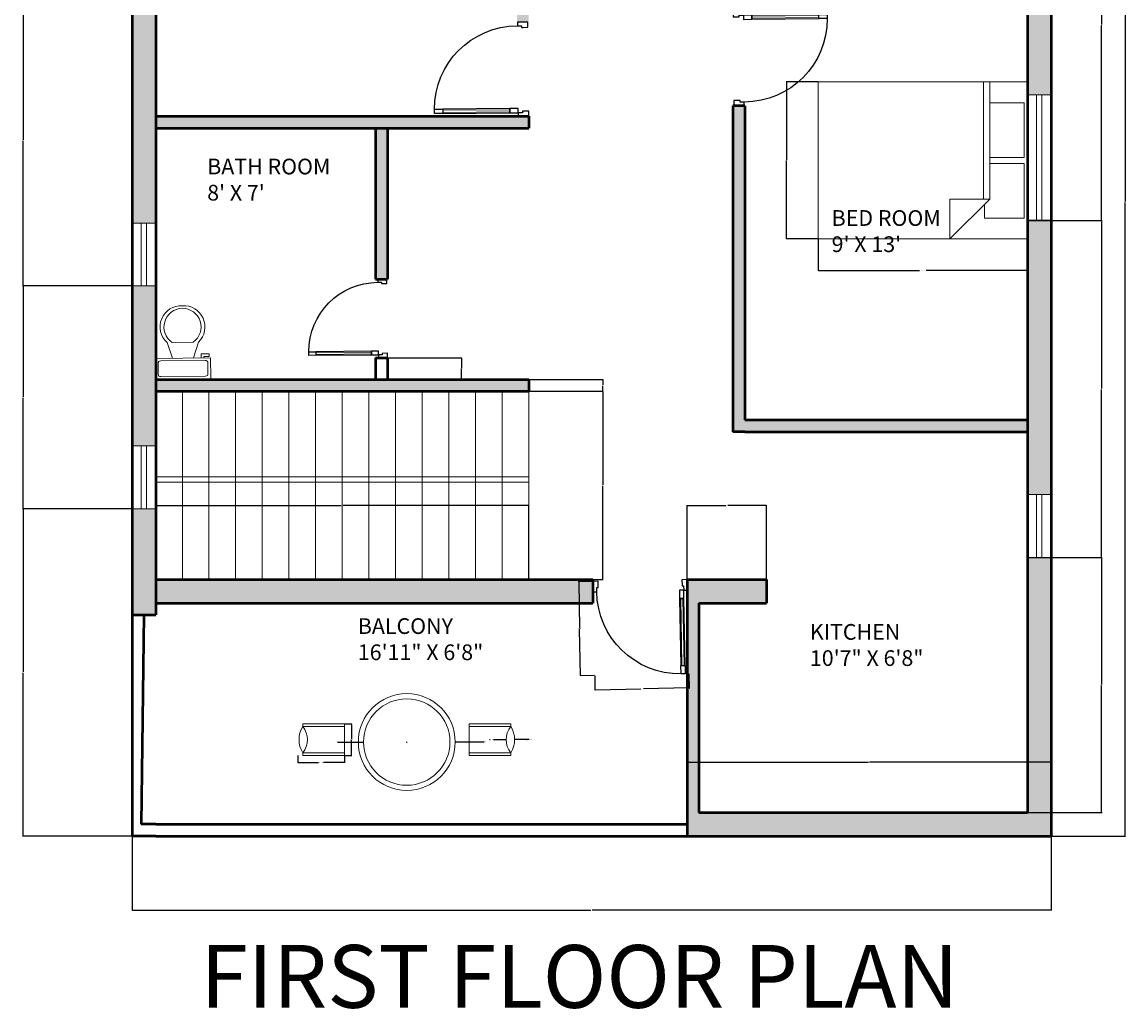
# Model space of a CAD drawing. Units: inches. Extents: x 5704 to 6126, y 2544 to 3123.
# Tile 1 of 2: x 5704 to 6126, y 2544 to 2921. Entities that reach past the tile are written whole.
import ezdxf

# ---------------------------------------------------------------- set-up
doc = ezdxf.new("R2010")
doc.units = ezdxf.units.IN
for name, color, linetype, lineweight in [('A-ANNO-DIMS', 2, 'Continuous', 18), ('A-ANNO-TEXT', 7, 'Continuous', 35), ('A-AREA-IDEN', 7, 'Continuous', 18), ('A-Door', 150, 'Continuous', 25), ('A-FLOR-FIXT', 9, 'Continuous', 18), ('A-FLOR-STRS', 7, 'Continuous', 18), ('A-FURN', 8, 'Continuous', 18), ('A-Glaz', 92, 'Continuous', 18), ('A-WALL', 7, 'Continuous', 50)]:
    doc.layers.add(name, color=color, linetype=linetype, lineweight=lineweight)
doc.layers.add('A-WALL-PATT', color=18, linetype='Continuous', lineweight=13, true_color=0x000000)
doc.styles.get("Standard").update_dxf_attribs({"font": 'arial.ttf'})
doc.dimstyles.get("Standard").update_dxf_attribs({"dimtxt": 0.18, "dimasz": 0.18, "dimexe": 0.18, "dimexo": 0.0625, "dimgap": 0.09, "dimtad": 0, "dimtih": 1, "dimtoh": 1, "dimdec": 4, "dimzin": 0, "dimdsep": 46, "dimtxsty": 'Standard', "dimcen": 0.09, "dimadec": 0, "dimazin": 0, "dimtfac": 1, "dimtdec": 4, "dimtofl": 0, "dimtmove": 0, "dimatfit": 3, "dimfxl": 1, "dimtolj": 1, "dimtzin": 0, "dimarcsym": 0})

# ---------------------------------------------------------------- blocks, each defined once
blk = doc.blocks.new('A$C61230BBC')
blk.add_lwpolyline([(825, 180), (825, 820), (865, 820), (865, 180)], close=True)
blk.add_arc((830, 105), 795, 90.3603, 180.3603)
at = {"layer": 'A-Door'}
for points in [[(825, 900), (825, 820), (865, 820), (865, 900)], [(825, 100), (825, 180), (865, 180), (865, 100)], [(35, 100), (35, 60), (50, 60), (50, 50), (50, 0), (0, 0), (0, 100)], [(865, 100), (900, 100), (900, 0), (850, 0), (850, 50), (850, 60), (865, 60)]]:
    blk.add_lwpolyline(points, close=True, dxfattribs=at)
at = {"layer": 'A-Glaz'}
blk.add_lwpolyline([(835, 180), (835, 820), (855, 820), (855, 180)], close=True, dxfattribs=at)
blk = doc.blocks.new('*U3')
for p, q in [((9.5, -6), (9.5, -2)), ((-8, -8.5), (-8, -8)), ((-7, -8), (-7, -9.5)), ((-4, -8), (-6, -14)), ((4, -8), (6, -14)), ((-10, -8.5), (-8, -8.5)), ((-10, -9.5), (-10, -8.5)), ((-7, -9.5), (-10, -9.5)), ((4, -14), (-4, -14))]:
    blk.add_line(p, q)
blk.add_lwpolyline([(10.5, -8), (10.5, 0), (-10.5, 0), (-10.5, -8)], close=True)
for points in [[(-9.5, -2), (-9.5, -6)], [(8.5, -1), (-8.5, -1)], [(-8.5, -7), (8.5, -7)]]:
    blk.add_lwpolyline(points)
for centre, radius, start, end in [((-8.625, -1.875), 0.8839, 81.8699, 188.1301), ((8.625, -1.875), 0.8839, 351.8699, 98.1301), ((-8.625, -6.125), 0.8839, 171.869898, 278.1301), ((8.625, -6.125), 0.8839, 261.8699, 8.1301), ((-0.4772, -19.9188), 8.0953, 133.01722, 273.38), ((0.0374, -19.8731), 7.127, 124.50543, 269.7), ((-0.0373, -19.8731), 7.127, 270.3, 55.4946), ((0.4773, -19.9188), 8.0953, 266.62, 46.9828)]:
    blk.add_arc(centre, radius, start, end)
blk = doc.blocks.new('Bed - Queen')
for p, q in [((0, -80.00003), (0, 0)), ((0, 0), (59.99999, 0)), ((59.99999, 0), (59.99999, -80.00003)), ((7.99999, -1.2), (28.79998, -1.2)), ((7.99999, -14.4), (7.99999, -1.2)), ((28.79998, -1.2), (28.79998, -14.4)), ((31.19999, -1.2), (51.99999, -1.2)), ((31.19999, -14.4), (31.19999, -1.2)), ((51.99999, -1.2), (51.99999, -16.4)), ((0, -14.4), (44.8, -14.4)), ((44.8, -16.8), (0, -16.8)), ((59.99999, -29.6), (44.8, -14.4)), ((44.8, -14.4), (44.8, -29.6)), ((51.99999, -16.4), (46.79936, -16.4)), ((44.8, -29.6), (59.99999, -29.6)), ((59.99999, -80.00003), (0, -80.00003))]:
    blk.add_line(p, q)
blk = doc.blocks.new('WIN-24IN')
for p, q in [((0, 9), (0, 0)), ((24, 9), (24, 0)), ((0, 5.5), (24, 5.5)), ((0, 3.5), (24, 3.5))]:
    blk.add_line(p, q)
blk = doc.blocks.new('WIN-48IN')
for p, q in [((0, 48), (9, 48)), ((3.5, 48), (3.5, 0)), ((5.5, 48), (5.5, 0)), ((5.5, 48), (5.5, 0)), ((0, 0), (9, 0))]:
    blk.add_line(p, q)
blk = doc.blocks.new('CHAIR-BALCONY')
for p, q in [((0, 12), (15.92, 12)), ((0, 12), (0, 0)), ((15.92, 11), (0, 11)), ((15.92, 12), (15.92, 11)), ((0, 1), (15.92, 1)), ((15.92, 0), (0, 0)), ((15.92, 1), (15.92, 0))]:
    blk.add_line(p, q)
for centre, radius, start, end in [((22.11, 6), 7.96, 141.1063, 218.8937), ((7.96, 6), 9.4, 327.8579, 32.1421)]:
    blk.add_arc(centre, radius, start, end)
blk = doc.blocks.new('*D10')
at = {"layer": 'A-ANNO-DIMS', "color": 0, "lineweight": -2, "transparency": 16777216}
for p, q in [((5922.38, 2706.94), (5916.86, 2706.84)), ((5917.05, 2706.66), (5917.38, 2689.03)), ((5917.72, 2671.03), (5917.38, 2688.66)), ((5923.06, 2670.95), (5917.54, 2670.85))]:
    blk.add_line(p, q, dxfattribs=at)
at = {"layer": 'A-ANNO-DIMS', "color": 0, "transparency": 16777216}
for points in [[(5917.08, 2706.66), (5917.02, 2706.66), (5917.04, 2706.84)], [(5917.75, 2671.03), (5917.69, 2671.03), (5917.72, 2670.85)]]:
    blk.add_solid(points, dxfattribs=at)
at = {"layer": 'Defpoints', "color": 0, "transparency": 16777216}
for p in [(5922.44, 2706.94), (5917.72, 2670.85), (5923.12, 2670.95)]:
    blk.add_point(p, dxfattribs=at)
at = {"layer": 'A-ANNO-DIMS', "color": 0, "transparency": 16777216, "insert": (5917.38, 2688.85), "char_height": 0.18, "attachment_point": 5}
blk.add_mtext('\\A1;DOOR 36 TYP.', dxfattribs=at)
blk = doc.blocks.new('*D11')
at = {"layer": 'A-ANNO-DIMS', "color": 0, "lineweight": -2, "transparency": 16777216}
for p, q in [((5923.12, 2670.89), (5923.22, 2665.37)), ((5959.11, 2671.56), (5959.22, 2666.05)), ((5923.4, 2665.55), (5940.69, 2665.88)), ((5959.03, 2666.22), (5941.74, 2665.9))]:
    blk.add_line(p, q, dxfattribs=at)
at = {"layer": 'A-ANNO-DIMS', "color": 0, "transparency": 16777216}
for points in [[(5923.4, 2665.58), (5923.4, 2665.52), (5923.22, 2665.55)], [(5959.03, 2666.25), (5959.03, 2666.19), (5959.21, 2666.23)]]:
    blk.add_solid(points, dxfattribs=at)
at = {"layer": 'Defpoints', "color": 0, "transparency": 16777216}
for p in [(5923.12, 2670.95), (5959.11, 2671.62), (5959.21, 2666.23)]:
    blk.add_point(p, dxfattribs=at)
at = {"layer": 'A-ANNO-DIMS', "color": 0, "transparency": 16777216, "insert": (5941.22, 2665.89), "char_height": 0.18, "attachment_point": 5}
blk.add_mtext('\\A1;36 TYP.', dxfattribs=at)
blk = doc.blocks.new('*D16')
at = {"layer": 'A-ANNO-DIMS', "color": 0, "lineweight": -2, "transparency": 16777216}
for p, q in [((6008.44, 2837.68), (6008.44, 2825.56)), ((6088.44, 2837.68), (6088.44, 2825.56)), ((6008.62, 2825.74), (6047.13, 2825.74)), ((6088.26, 2825.74), (6049.74, 2825.74))]:
    blk.add_line(p, q, dxfattribs=at)
at = {"layer": 'A-ANNO-DIMS', "color": 0, "transparency": 16777216}
for points in [[(6008.62, 2825.77), (6008.62, 2825.71), (6008.44, 2825.74)], [(6088.26, 2825.77), (6088.26, 2825.71), (6088.44, 2825.74)]]:
    blk.add_solid(points, dxfattribs=at)
at = {"layer": 'Defpoints', "color": 0, "transparency": 16777216}
for p in [(6008.44, 2837.74), (6088.44, 2837.74), (6088.44, 2825.74)]:
    blk.add_point(p, dxfattribs=at)
at = {"layer": 'A-ANNO-DIMS', "color": 0, "transparency": 16777216, "insert": (6048.44, 2825.74), "char_height": 0.18, "attachment_point": 5}
blk.add_mtext('\\A1;QUEEN BED 80 TYP.', dxfattribs=at)
blk = doc.blocks.new('*D17')
at = {"layer": 'A-ANNO-DIMS', "color": 0, "lineweight": -2, "transparency": 16777216}
for p, q in [((6008.37, 2897.74), (5996.26, 2897.74)), ((5996.44, 2897.56), (5996.44, 2867.92)), ((5996.44, 2837.92), (5996.44, 2867.56)), ((6008.37, 2837.74), (5996.26, 2837.74))]:
    blk.add_line(p, q, dxfattribs=at)
at = {"layer": 'A-ANNO-DIMS', "color": 0, "transparency": 16777216}
for points in [[(5996.41, 2897.56), (5996.47, 2897.56), (5996.44, 2897.74)], [(5996.41, 2837.92), (5996.47, 2837.92), (5996.44, 2837.74)]]:
    blk.add_solid(points, dxfattribs=at)
at = {"layer": 'Defpoints', "color": 0, "transparency": 16777216}
for p in [(6008.44, 2897.74), (5996.44, 2837.74), (6008.44, 2837.74)]:
    blk.add_point(p, dxfattribs=at)
at = {"layer": 'A-ANNO-DIMS', "color": 0, "transparency": 16777216, "insert": (5996.44, 2867.74), "char_height": 0.18, "attachment_point": 5}
blk.add_mtext('\\A1;60 TYP.', dxfattribs=at)
blk = doc.blocks.new('*D18')
at = {"layer": 'A-ANNO-DIMS', "color": 0, "lineweight": -2, "transparency": 16777216}
for p, q in [((5809.71, 2640.4), (5809.71, 2637.6)), ((5827.55, 2640.4), (5827.55, 2637.6)), ((5809.89, 2637.78), (5817.68, 2637.78)), ((5827.37, 2637.78), (5819.58, 2637.78))]:
    blk.add_line(p, q, dxfattribs=at)
at = {"layer": 'A-ANNO-DIMS', "color": 0, "transparency": 16777216}
for points in [[(5809.89, 2637.81), (5809.89, 2637.75), (5809.71, 2637.78)], [(5827.37, 2637.81), (5827.37, 2637.75), (5827.55, 2637.78)]]:
    blk.add_solid(points, dxfattribs=at)
at = {"layer": 'Defpoints', "color": 0, "transparency": 16777216}
for p in [(5809.71, 2640.46), (5827.55, 2640.46), (5809.71, 2637.78)]:
    blk.add_point(p, dxfattribs=at)
at = {"layer": 'A-ANNO-DIMS', "color": 0, "transparency": 16777216, "insert": (5818.63, 2637.78), "char_height": 0.18, "attachment_point": 5}
blk.add_mtext('\\A1;CHAIR 18 TYP.', dxfattribs=at)
blk = doc.blocks.new('*D19')
at = {"layer": 'A-ANNO-DIMS', "color": 0, "lineweight": -2, "transparency": 16777216}
for p, q in [((5827.61, 2652.46), (5830.4, 2652.46)), ((5830.22, 2652.28), (5830.22, 2646.64)), ((5830.22, 2640.64), (5830.22, 2646.28)), ((5827.61, 2640.46), (5830.4, 2640.46))]:
    blk.add_line(p, q, dxfattribs=at)
at = {"layer": 'A-ANNO-DIMS', "color": 0, "transparency": 16777216}
for points in [[(5830.19, 2652.28), (5830.25, 2652.28), (5830.22, 2652.46)], [(5830.19, 2640.64), (5830.25, 2640.64), (5830.22, 2640.46)]]:
    blk.add_solid(points, dxfattribs=at)
at = {"layer": 'Defpoints', "color": 0, "transparency": 16777216}
for p in [(5827.55, 2652.46), (5827.55, 2640.46), (5830.22, 2640.46)]:
    blk.add_point(p, dxfattribs=at)
at = {"layer": 'A-ANNO-DIMS', "color": 0, "transparency": 16777216, "insert": (5830.22, 2646.46), "char_height": 0.18, "attachment_point": 5}
blk.add_mtext('\\A1;12 TYP.', dxfattribs=at)
blk = doc.blocks.new('*D20')
at = {"layer": 'A-ANNO-DIMS', "color": 0, "lineweight": -2, "transparency": 16777216}
for p, q in [((5746.436687, 2609.555742), (5746.436687, 2581.138242)), ((6097.436687, 2609.555742), (6097.436687, 2581.138242)), ((5746.616687, 2581.318242), (5921.665275, 2581.318242)), ((6097.256687, 2581.318242), (5922.208099, 2581.318242))]:
    blk.add_line(p, q, dxfattribs=at)
at = {"layer": 'A-ANNO-DIMS', "color": 0, "transparency": 16777216}
for points in [[(5746.616687, 2581.348242), (5746.616687, 2581.288242), (5746.436687, 2581.318242)], [(6097.256687, 2581.348242), (6097.256687, 2581.288242), (6097.436687, 2581.318242)]]:
    blk.add_solid(points, dxfattribs=at)
at = {"layer": 'Defpoints', "color": 0, "transparency": 16777216}
for p in [(5746.436687, 2609.618242), (6097.436687, 2609.618242), (6097.436687, 2581.318242)]:
    blk.add_point(p, dxfattribs=at)
at = {"layer": 'A-ANNO-DIMS', "color": 0, "transparency": 16777216, "insert": (5921.936687, 2581.318242), "char_height": 0.18, "attachment_point": 5}
blk.add_mtext('\\A1;351', dxfattribs=at)
blk = doc.blocks.new('*D21')
at = {"layer": 'A-ANNO-DIMS', "color": 0, "lineweight": -2, "transparency": 16777216}
for p, q in [((6097.5, 3094.12), (6125.92, 3094.12)), ((6125.74, 3093.94), (6125.74, 2852.05)), ((6125.74, 2609.8), (6125.74, 2851.69)), ((6097.5, 2609.62), (6125.92, 2609.62))]:
    blk.add_line(p, q, dxfattribs=at)
at = {"layer": 'A-ANNO-DIMS', "color": 0, "transparency": 16777216}
for points in [[(6125.71, 3093.94), (6125.77, 3093.94), (6125.74, 3094.12)], [(6125.71, 2609.8), (6125.77, 2609.8), (6125.74, 2609.62)]]:
    blk.add_solid(points, dxfattribs=at)
at = {"layer": 'Defpoints', "color": 0, "transparency": 16777216}
for p in [(6097.44, 3094.12), (6125.74, 3094.12), (6097.44, 2609.62)]:
    blk.add_point(p, dxfattribs=at)
at = {"layer": 'A-ANNO-DIMS', "color": 0, "transparency": 16777216, "insert": (6125.74, 2851.87), "char_height": 0.18, "attachment_point": 5}
blk.add_mtext('\\A1;484.5', dxfattribs=at)
blk = doc.blocks.new('*D24')
at = {"layer": 'A-ANNO-DIMS', "color": 0, "lineweight": -2, "transparency": 16777216}
for p, q in [((5746.37, 2734.68), (5704.59, 2734.68)), ((5704.77, 2734.5), (5704.77, 2672.33)), ((5704.77, 2609.8), (5704.77, 2671.97)), ((5746.37, 2609.62), (5704.59, 2609.62))]:
    blk.add_line(p, q, dxfattribs=at)
at = {"layer": 'A-ANNO-DIMS', "color": 0, "transparency": 16777216}
for points in [[(5704.74, 2734.5), (5704.8, 2734.5), (5704.77, 2734.68)], [(5704.74, 2609.8), (5704.8, 2609.8), (5704.77, 2609.62)]]:
    blk.add_solid(points, dxfattribs=at)
at = {"layer": 'Defpoints', "color": 0, "transparency": 16777216}
for p in [(5704.77, 2734.68), (5746.44, 2734.68), (5746.44, 2609.62)]:
    blk.add_point(p, dxfattribs=at)
at = {"layer": 'A-ANNO-DIMS', "color": 0, "transparency": 16777216, "insert": (5704.77, 2672.15), "char_height": 0.18, "attachment_point": 5}
blk.add_mtext('\\A1;125.06', dxfattribs=at)
blk = doc.blocks.new('*D25')
at = {"layer": 'A-ANNO-DIMS', "color": 0, "lineweight": -2, "transparency": 16777216}
for p, q in [((5746.37, 2819.8), (5704.59, 2819.8)), ((5704.77, 2819.62), (5704.77, 2777.42)), ((5704.77, 2734.86), (5704.77, 2777.06)), ((5746.37, 2734.68), (5704.59, 2734.68))]:
    blk.add_line(p, q, dxfattribs=at)
at = {"layer": 'A-ANNO-DIMS', "color": 0, "transparency": 16777216}
for points in [[(5704.74, 2819.62), (5704.8, 2819.62), (5704.77, 2819.8)], [(5704.74, 2734.86), (5704.8, 2734.86), (5704.77, 2734.68)]]:
    blk.add_solid(points, dxfattribs=at)
at = {"layer": 'Defpoints', "color": 0, "transparency": 16777216}
for p in [(5704.77, 2819.8), (5746.44, 2819.8), (5746.44, 2734.68)]:
    blk.add_point(p, dxfattribs=at)
at = {"layer": 'A-ANNO-DIMS', "color": 0, "transparency": 16777216, "insert": (5704.77, 2777.24), "char_height": 0.18, "attachment_point": 5}
blk.add_mtext('\\A1;85.12', dxfattribs=at)
blk = doc.blocks.new('*D26')
at = {"layer": 'A-ANNO-DIMS', "color": 0, "lineweight": -2, "transparency": 16777216}
for p, q in [((5746.37, 2931.06), (5704.59, 2931.06)), ((5704.77, 2930.88), (5704.77, 2875.61)), ((5704.77, 2819.98), (5704.77, 2875.25)), ((5746.37, 2819.8), (5704.59, 2819.8))]:
    blk.add_line(p, q, dxfattribs=at)
at = {"layer": 'A-ANNO-DIMS', "color": 0, "transparency": 16777216}
for points in [[(5704.74, 2930.88), (5704.8, 2930.88), (5704.77, 2931.06)], [(5704.74, 2819.98), (5704.8, 2819.98), (5704.77, 2819.8)]]:
    blk.add_solid(points, dxfattribs=at)
at = {"layer": 'Defpoints', "color": 0, "transparency": 16777216}
for p in [(5704.77, 2931.06), (5746.44, 2931.06), (5746.44, 2819.8)]:
    blk.add_point(p, dxfattribs=at)
at = {"layer": 'A-ANNO-DIMS', "color": 0, "transparency": 16777216, "insert": (5704.77, 2875.43), "char_height": 0.18, "attachment_point": 5}
blk.add_mtext('\\A1;111.27', dxfattribs=at)
blk = doc.blocks.new('*D27')
at = {"layer": 'A-ANNO-DIMS', "color": 0, "lineweight": -2, "transparency": 16777216}
for p, q in [((6088.5, 2716.09), (6116.92, 2716.09)), ((6116.74, 2715.91), (6116.74, 2667.54)), ((6116.74, 2618.8), (6116.74, 2667.17)), ((6088.5, 2618.62), (6116.92, 2618.62))]:
    blk.add_line(p, q, dxfattribs=at)
at = {"layer": 'A-ANNO-DIMS', "color": 0, "transparency": 16777216}
for points in [[(6116.71, 2715.91), (6116.77, 2715.91), (6116.74, 2716.09)], [(6116.71, 2618.8), (6116.77, 2618.8), (6116.74, 2618.62)]]:
    blk.add_solid(points, dxfattribs=at)
at = {"layer": 'Defpoints', "color": 0, "transparency": 16777216}
for p in [(6088.44, 2716.09), (6088.44, 2618.62), (6116.74, 2618.62)]:
    blk.add_point(p, dxfattribs=at)
at = {"layer": 'A-ANNO-DIMS', "color": 0, "transparency": 16777216, "insert": (6116.74, 2667.36), "char_height": 0.18, "attachment_point": 5}
blk.add_mtext('\\A1;97.48', dxfattribs=at)
blk = doc.blocks.new('*D28')
at = {"layer": 'A-ANNO-DIMS', "color": 0, "lineweight": -2, "transparency": 16777216}
for p, q in [((6088.5, 2844.87), (6116.92, 2844.87)), ((6116.74, 2844.69), (6116.74, 2780.66)), ((6116.74, 2716.27), (6116.74, 2780.3)), ((6088.5, 2716.09), (6116.92, 2716.09))]:
    blk.add_line(p, q, dxfattribs=at)
at = {"layer": 'A-ANNO-DIMS', "color": 0, "transparency": 16777216}
for points in [[(6116.71, 2844.69), (6116.77, 2844.69), (6116.74, 2844.87)], [(6116.71, 2716.27), (6116.77, 2716.27), (6116.74, 2716.09)]]:
    blk.add_solid(points, dxfattribs=at)
at = {"layer": 'Defpoints', "color": 0, "transparency": 16777216}
for p in [(6088.44, 2844.87), (6088.44, 2716.09), (6116.74, 2716.09)]:
    blk.add_point(p, dxfattribs=at)
at = {"layer": 'A-ANNO-DIMS', "color": 0, "transparency": 16777216, "insert": (6116.74, 2780.48), "char_height": 0.18, "attachment_point": 5}
blk.add_mtext('\\A1;128.78', dxfattribs=at)
blk = doc.blocks.new('*D29')
at = {"layer": 'A-ANNO-DIMS', "color": 0, "lineweight": -2, "transparency": 16777216}
for p, q in [((6088.5, 2994.02), (6116.92, 2994.02)), ((6116.74, 2993.84), (6116.74, 2919.63)), ((6116.74, 2845.05), (6116.74, 2919.26)), ((6088.5, 2844.87), (6116.92, 2844.87))]:
    blk.add_line(p, q, dxfattribs=at)
at = {"layer": 'A-ANNO-DIMS', "color": 0, "transparency": 16777216}
for points in [[(6116.71, 2993.84), (6116.77, 2993.84), (6116.74, 2994.02)], [(6116.71, 2845.05), (6116.77, 2845.05), (6116.74, 2844.87)]]:
    blk.add_solid(points, dxfattribs=at)
at = {"layer": 'Defpoints', "color": 0, "transparency": 16777216}
for p in [(6088.44, 2994.02), (6088.44, 2844.87), (6116.74, 2844.87)]:
    blk.add_point(p, dxfattribs=at)
at = {"layer": 'A-ANNO-DIMS', "color": 0, "transparency": 16777216, "insert": (6116.74, 2919.45), "char_height": 0.18, "attachment_point": 5}
blk.add_mtext('\\A1;149.15', dxfattribs=at)
blk = doc.blocks.new('*D30')
at = {"layer": 'A-ANNO-DIMS', "color": 0, "lineweight": -2, "transparency": 16777216}
for p, q in [((5898, 2784.12), (5926.42, 2784.12)), ((5926.24, 2783.94), (5926.24, 2782.05)), ((5898, 2779.62), (5926.42, 2779.62)), ((5926.24, 2779.8), (5926.24, 2781.69))]:
    blk.add_line(p, q, dxfattribs=at)
at = {"layer": 'A-ANNO-DIMS', "color": 0, "transparency": 16777216}
for points in [[(5926.21, 2783.94), (5926.27, 2783.94), (5926.24, 2784.12)], [(5926.21, 2779.8), (5926.27, 2779.8), (5926.24, 2779.62)]]:
    blk.add_solid(points, dxfattribs=at)
at = {"layer": 'Defpoints', "color": 0, "transparency": 16777216}
for p in [(5897.94, 2784.12), (5897.94, 2779.62), (5926.24, 2779.62)]:
    blk.add_point(p, dxfattribs=at)
at = {"layer": 'A-ANNO-DIMS', "color": 0, "transparency": 16777216, "insert": (5926.24, 2781.87), "char_height": 0.18, "attachment_point": 5}
blk.add_mtext('\\A1;4.5', dxfattribs=at)
blk = doc.blocks.new('*D32')
at = {"layer": 'A-ANNO-DIMS', "color": 0, "lineweight": -2, "transparency": 16777216}
for p, q in [((5898, 2779.62), (5926.42, 2779.62)), ((5926.24, 2779.44), (5926.24, 2743.8)), ((5926.24, 2707.8), (5926.24, 2743.44)), ((5898, 2707.62), (5926.42, 2707.62))]:
    blk.add_line(p, q, dxfattribs=at)
at = {"layer": 'A-ANNO-DIMS', "color": 0, "transparency": 16777216}
for points in [[(5926.21, 2779.44), (5926.27, 2779.44), (5926.24, 2779.62)], [(5926.21, 2707.8), (5926.27, 2707.8), (5926.24, 2707.62)]]:
    blk.add_solid(points, dxfattribs=at)
at = {"layer": 'Defpoints', "color": 0, "transparency": 16777216}
for p in [(5897.94, 2779.62), (5897.94, 2707.62), (5926.24, 2707.62)]:
    blk.add_point(p, dxfattribs=at)
at = {"layer": 'A-ANNO-DIMS', "color": 0, "transparency": 16777216, "insert": (5926.24, 2743.62), "char_height": 0.18, "attachment_point": 5}
blk.add_mtext('\\A1;72', dxfattribs=at)
blk = doc.blocks.new('*D33')
at = {"layer": 'A-ANNO-DIMS', "color": 0, "lineweight": -2, "transparency": 16777216}
for p, q in [((5755.44, 2707.68), (5755.44, 2736.1)), ((5755.62, 2735.92), (5826.3, 2735.92)), ((5897.76, 2735.92), (5827.07, 2735.92)), ((5897.94, 2707.68), (5897.94, 2736.1))]:
    blk.add_line(p, q, dxfattribs=at)
at = {"layer": 'A-ANNO-DIMS', "color": 0, "transparency": 16777216}
for points in [[(5755.62, 2735.95), (5755.62, 2735.89), (5755.44, 2735.92)], [(5897.76, 2735.95), (5897.76, 2735.89), (5897.94, 2735.92)]]:
    blk.add_solid(points, dxfattribs=at)
at = {"layer": 'Defpoints', "color": 0, "transparency": 16777216}
for p in [(5897.94, 2735.92), (5755.44, 2707.62), (5897.94, 2707.62)]:
    blk.add_point(p, dxfattribs=at)
at = {"layer": 'A-ANNO-DIMS', "color": 0, "transparency": 16777216, "insert": (5826.69, 2735.92), "char_height": 0.18, "attachment_point": 5}
blk.add_mtext('\\A1;142.5', dxfattribs=at)
blk = doc.blocks.new('*D34')
at = {"layer": 'A-ANNO-DIMS', "color": 0, "lineweight": -2, "transparency": 16777216}
for p, q in [((5844, 2792.4), (5872.42, 2792.4)), ((5872.24, 2792.22), (5872.24, 2788.44)), ((5872.24, 2784.3), (5872.24, 2788.08)), ((5844, 2784.12), (5872.42, 2784.12))]:
    blk.add_line(p, q, dxfattribs=at)
at = {"layer": 'A-ANNO-DIMS', "color": 0, "transparency": 16777216}
for points in [[(5872.21, 2792.22), (5872.27, 2792.22), (5872.24, 2792.4)], [(5872.21, 2784.3), (5872.27, 2784.3), (5872.24, 2784.12)]]:
    blk.add_solid(points, dxfattribs=at)
at = {"layer": 'Defpoints', "color": 0, "transparency": 16777216}
for p in [(5843.94, 2792.4), (5843.94, 2784.12), (5872.24, 2784.12)]:
    blk.add_point(p, dxfattribs=at)
at = {"layer": 'A-ANNO-DIMS', "color": 0, "transparency": 16777216, "insert": (5872.24, 2788.26), "char_height": 0.18, "attachment_point": 5}
blk.add_mtext('\\A1;8.278', dxfattribs=at)
blk = doc.blocks.new('*D35')
at = {"layer": 'A-ANNO-DIMS', "color": 0, "lineweight": -2, "transparency": 16777216}
for p, q in [((5958.44, 2609.68), (5958.44, 2638.1)), ((5958.62, 2637.92), (6027.66, 2637.92)), ((6097.26, 2637.92), (6028.22, 2637.92)), ((6097.44, 2609.68), (6097.44, 2638.1))]:
    blk.add_line(p, q, dxfattribs=at)
at = {"layer": 'A-ANNO-DIMS', "color": 0, "transparency": 16777216}
for points in [[(5958.62, 2637.95), (5958.62, 2637.89), (5958.44, 2637.92)], [(6097.26, 2637.95), (6097.26, 2637.89), (6097.44, 2637.92)]]:
    blk.add_solid(points, dxfattribs=at)
at = {"layer": 'Defpoints', "color": 0, "transparency": 16777216}
for p in [(6097.44, 2637.92), (5958.44, 2609.62), (6097.44, 2609.62)]:
    blk.add_point(p, dxfattribs=at)
at = {"layer": 'A-ANNO-DIMS', "color": 0, "transparency": 16777216, "insert": (6027.94, 2637.92), "char_height": 0.18, "attachment_point": 5}
blk.add_mtext('\\A1;139', dxfattribs=at)
blk = doc.blocks.new('*D36')
at = {"layer": 'A-ANNO-DIMS', "color": 0, "lineweight": -2, "transparency": 16777216}
for p, q in [((5958.44, 2707.68), (5958.44, 2736.1)), ((5958.62, 2735.92), (5973.22, 2735.92)), ((5988.61, 2735.92), (5974.01, 2735.92)), ((5988.79, 2707.68), (5988.79, 2736.1))]:
    blk.add_line(p, q, dxfattribs=at)
at = {"layer": 'A-ANNO-DIMS', "color": 0, "transparency": 16777216}
for points in [[(5958.62, 2735.95), (5958.62, 2735.89), (5958.44, 2735.92)], [(5988.61, 2735.95), (5988.61, 2735.89), (5988.79, 2735.92)]]:
    blk.add_solid(points, dxfattribs=at)
at = {"layer": 'Defpoints', "color": 0, "transparency": 16777216}
for p in [(5988.79, 2735.92), (5958.44, 2707.62), (5988.79, 2707.62)]:
    blk.add_point(p, dxfattribs=at)
at = {"layer": 'A-ANNO-DIMS', "color": 0, "transparency": 16777216, "insert": (5973.62, 2735.92), "char_height": 0.18, "attachment_point": 5}
blk.add_mtext('\\A1;30.36', dxfattribs=at)
blk = doc.blocks.new('*D37')
at = {"layer": 'A-ANNO-DIMS', "color": 0, "lineweight": -2, "transparency": 16777216}
for p, q in [((5851.25, 2645.55), (5851.43, 2645.55)), ((5851.34, 2645.46), (5851.34, 2645.64)), ((5880.94, 2645.55), (5870.02, 2645.55))]:
    blk.add_line(p, q, dxfattribs=at)
at = {"layer": 'A-ANNO-DIMS', "color": 0, "transparency": 16777216}
blk.add_solid([(5870.02, 2645.58), (5870.02, 2645.52), (5869.84, 2645.55)], dxfattribs=at)
at = {"layer": 'Defpoints', "color": 0, "transparency": 16777216}
for p in [(5832.84, 2645.55), (5869.84, 2645.55)]:
    blk.add_point(p, dxfattribs=at)
at = {"layer": 'A-ANNO-DIMS', "color": 0, "transparency": 16777216, "insert": (5881.26, 2645.55), "char_height": 0.18, "attachment_point": 5}
blk.add_mtext('\\A1;∅37', dxfattribs=at)
blk = doc.blocks.new('*D38')
at = {"layer": 'A-ANNO-DIMS', "color": 0, "lineweight": -2, "transparency": 16777216}
for p, q in [((5824.94, 2645.55), (5834.66, 2645.55)), ((5851.25, 2645.55), (5851.43, 2645.55)), ((5851.34, 2645.46), (5851.34, 2645.64))]:
    blk.add_line(p, q, dxfattribs=at)
at = {"layer": 'A-ANNO-DIMS', "color": 0, "transparency": 16777216}
blk.add_solid([(5834.66, 2645.58), (5834.66, 2645.52), (5834.84, 2645.55)], dxfattribs=at)
at = {"layer": 'Defpoints', "color": 0, "transparency": 16777216}
for p in [(5834.84, 2645.55), (5867.84, 2645.55)]:
    blk.add_point(p, dxfattribs=at)
at = {"layer": 'A-ANNO-DIMS', "color": 0, "transparency": 16777216, "insert": (5824.62, 2645.55), "char_height": 0.18, "attachment_point": 5}
blk.add_mtext('\\A1;∅33', dxfattribs=at)
blk = doc.blocks.new('*D39')
at = {"layer": 'A-ANNO-DIMS', "color": 0, "lineweight": -2, "transparency": 16777216}
for p, q in [((5883.03, 2646.46), (5883.21, 2646.46)), ((5883.12, 2646.37), (5883.12, 2646.55)), ((5898.15, 2646.46), (5892.69, 2646.46))]:
    blk.add_line(p, q, dxfattribs=at)
at = {"layer": 'A-ANNO-DIMS', "color": 0, "transparency": 16777216}
blk.add_solid([(5892.69, 2646.49), (5892.69, 2646.43), (5892.51, 2646.46)], dxfattribs=at)
at = {"layer": 'Defpoints', "color": 0, "transparency": 16777216}
for p in [(5883.12, 2646.46), (5892.51, 2646.46)]:
    blk.add_point(p, dxfattribs=at)
at = {"layer": 'A-ANNO-DIMS', "color": 0, "transparency": 16777216, "insert": (5898.83, 2646.46), "char_height": 0.18, "attachment_point": 5}
blk.add_mtext('\\A1;2X R9.398', dxfattribs=at)
blk = doc.blocks.new('*D40')
at = {"layer": 'A-ANNO-DIMS', "color": 0, "lineweight": -2, "transparency": 16777216}
for p, q in [((5884.53, 2646.46), (5889.13, 2646.46)), ((5897.18, 2646.46), (5897.36, 2646.46)), ((5897.27, 2646.37), (5897.27, 2646.55))]:
    blk.add_line(p, q, dxfattribs=at)
at = {"layer": 'A-ANNO-DIMS', "color": 0, "transparency": 16777216}
blk.add_solid([(5889.13, 2646.49), (5889.13, 2646.43), (5889.31, 2646.46)], dxfattribs=at)
at = {"layer": 'Defpoints', "color": 0, "transparency": 16777216}
for p in [(5889.31, 2646.46), (5897.27, 2646.46)]:
    blk.add_point(p, dxfattribs=at)
at = {"layer": 'A-ANNO-DIMS', "color": 0, "transparency": 16777216, "insert": (5883.86, 2646.46), "char_height": 0.18, "attachment_point": 5}
blk.add_mtext('\\A1;2X R7.963', dxfattribs=at)

msp = doc.modelspace()

# ---------------------------------------------------------------- hatches: boundary and pattern name
at = {"layer": 'A-WALL-PATT'}
h = msp.add_hatch(color=256, dxfattribs=at)
h.dxf.hatch_style = 1
h.paths.add_polyline_path([(5755.4367, 2734.6788), (5746.4367, 2734.6788), (5746.4367, 2694.1938), (5755.4367, 2694.1938)])
h.paths.add_polyline_path([(5755.4367, 2931.063), (5746.4367, 2931.063), (5746.4367, 2843.7971), (5755.4367, 2843.7971)])
h.paths.add_polyline_path([(5755.4367, 3094.1182), (5746.4367, 3094.1182), (5746.4367, 2979.063), (5755.4367, 2979.063)])
h.paths.add_polyline_path([(5810.5679, 3094.1182), (5755.4367, 3094.1182), (5755.4367, 3085.1182), (5810.5679, 3085.1182)])
h.paths.add_polyline_path([(5895.3146, 3094.1182), (5834.5679, 3094.1182), (5834.5679, 3085.1182), (5895.3146, 3085.1182)])
h.paths.add_polyline_path([(6097.4367, 3094.1182), (5919.3146, 3094.1182), (5919.3146, 3085.1182), (6088.4367, 3085.1182), (6088.4367, 3042.019), (6097.4367, 3042.019), (6097.4367, 3085.1182)])
h.paths.add_polyline_path([(6097.4367, 2994.019), (6088.4367, 2994.019), (6088.4367, 2892.8723), (6097.4367, 2892.8723)])
h.paths.add_polyline_path([(6097.4367, 2844.8723), (6088.4367, 2844.8723), (6088.4367, 2740.0934), (6097.4367, 2740.0934)])
h = msp.add_hatch(color=256, dxfattribs=at)
h.dxf.hatch_style = 1
h.paths.add_polyline_path([(5980.4367, 3055.1182), (5975.9367, 3055.1182), (5975.9367, 3015.1182), (5879.9367, 3015.1182), (5879.9367, 3085.1182), (5875.4367, 3085.1182), (5875.4367, 3010.6182), (5879.9367, 3010.6182), (5975.9367, 3010.6182), (5975.9367, 2965.1182), (5980.4367, 2965.1182)])
h.paths.add_polyline_path([(5897.9367, 3010.6182), (5893.4367, 3010.6182), (5893.4367, 2920.6182), (5897.9367, 2920.6182)])
h.paths.add_polyline_path([(5845.4367, 3015.1182), (5755.4367, 3015.1182), (5755.4367, 3010.6182), (5845.4367, 3010.6182)])
h.paths.add_polyline_path([(5897.9367, 2884.6182), (5845.4367, 2884.6182), (5755.4367, 2884.6182), (5755.4367, 2880.1182), (5845.4367, 2880.1182), (5897.9367, 2880.1182)])
h.paths.add_polyline_path([(5843.9367, 2880.1182), (5839.4367, 2880.1182), (5839.4367, 2822.3967), (5843.9367, 2822.3967)])
h.paths.add_polyline_path([(5922.4367, 2707.6182), (5897.9367, 2707.6182), (5845.4367, 2707.6182), (5755.4367, 2707.6182), (5755.4367, 2698.6182), (5845.4367, 2698.6182), (5897.9367, 2698.6182), (5922.4367, 2698.6182)])
h.paths.add_polyline_path([(5897.9367, 2784.1182), (5845.4367, 2784.1182), (5755.4367, 2784.1182), (5755.4367, 2779.6182), (5845.4367, 2779.6182), (5897.9367, 2779.6182)])
h = msp.add_hatch(color=256, dxfattribs=at)
h.dxf.hatch_style = 1
h.paths.add_polyline_path([(5988.7946, 2707.6182), (5958.4367, 2707.6182), (5958.5117, 2703.6189), (5958.4367, 2703.6175), (5958.4367, 2618.6182), (5958.4367, 2609.6182), (6097.4367, 2609.6182), (6097.4367, 2716.0934), (6088.4367, 2716.0934), (6088.4367, 2618.6182), (5962.9367, 2618.6182), (5962.9367, 2698.6182), (5988.7946, 2698.6182)])
h.paths.add_polyline_path([(5980.4367, 2888.6182), (5975.9367, 2888.6182), (5975.9367, 2764.1182), (5980.4367, 2764.1182), (6088.4367, 2764.1182), (6088.4367, 2768.6182), (5980.4367, 2768.6182)])
h.paths.add_polyline_path([(6088.4367, 2929.1182), (5980.4367, 2929.1182), (5975.9367, 2929.1182), (5975.9367, 2924.6182), (5980.4367, 2924.6182), (6088.4367, 2924.6182)])
h = msp.add_hatch(color=256, dxfattribs=at)
h.dxf.hatch_style = 1
h.paths.add_polyline_path([(5755.4367, 2784.1182), (5755.4367, 2819.7971), (5746.4367, 2819.7971), (5746.4367, 2758.6788), (5755.4367, 2758.6788)])

# ---------------------------------------------------------------- linework, layer by layer
at = {"layer": 'A-FLOR-STRS'}
for p, q in [((5755.4367, 2784.1182), (5755.4367, 2707.6182)), ((5897.9367, 2784.1182), (5897.9367, 2707.6182)), ((5765.6153, 2779.6182), (5765.6153, 2707.6182)), ((5775.7938, 2779.6182), (5775.7938, 2707.6182)), ((5785.9724, 2779.6182), (5785.9724, 2707.6182)), ((5796.151, 2779.6182), (5796.151, 2707.6182)), ((5806.3295, 2779.6182), (5806.3295, 2707.6182)), ((5816.5081, 2779.6182), (5816.5081, 2707.6182)), ((5826.6867, 2779.6182), (5826.6867, 2707.6182)), ((5836.8653, 2779.6182), (5836.8653, 2707.6182)), ((5847.0438, 2779.6182), (5847.0438, 2707.6182)), ((5857.2224, 2779.6182), (5857.2224, 2707.6182)), ((5867.401, 2779.6182), (5867.401, 2707.6182)), ((5877.5795, 2779.6182), (5877.5795, 2707.6182)), ((5887.7581, 2779.6182), (5887.7581, 2707.6182)), ((5897.9367, 2746.8682), (5755.4367, 2746.8682)), ((5897.9367, 2744.8682), (5755.4367, 2744.8682))]:
    msp.add_line(p, q, dxfattribs=at)
at = {"layer": 'A-FURN'}
for radius in [18.5016, 16.5016]:
    msp.add_circle((5851.3402, 2645.5521), radius, dxfattribs=at)
at = {"layer": 'A-WALL'}
for p, q in [((5746.4367, 3094.1182), (5746.4367, 2609.6182)), ((5755.4367, 3094.1182), (5755.4367, 2694.1938)), ((6088.4367, 3085.1182), (6088.4367, 2618.6182)), ((6097.4367, 3085.1182), (6097.4367, 2609.6182)), ((5980.4367, 2888.6182), (5975.9367, 2888.6182)), ((5975.9367, 2888.6182), (5975.9367, 2764.1182)), ((5980.4367, 2888.6182), (5980.4367, 2768.6182)), ((5755.4367, 2884.6182), (5845.4367, 2884.6182)), ((5845.4367, 2884.6182), (5897.9367, 2884.6182)), ((5897.9367, 2884.6182), (5897.9367, 2880.1182)), ((5755.4367, 2880.1182), (5845.4367, 2880.1182)), ((5839.4367, 2880.1182), (5839.4367, 2822.3967)), ((5843.9367, 2880.1182), (5843.9367, 2822.3967)), ((5845.4367, 2880.1182), (5897.9367, 2880.1182)), ((5839.4367, 2822.3967), (5843.9367, 2822.3967)), ((5839.4367, 2792.3967), (5843.9367, 2792.3967)), ((5839.4367, 2792.3967), (5839.4367, 2784.1182)), ((5843.9367, 2792.3967), (5843.9367, 2784.1182)), ((5755.4367, 2784.1182), (5845.4367, 2784.1182)), ((5845.4367, 2784.1182), (5897.9367, 2784.1182)), ((5897.9367, 2784.1182), (5897.9367, 2779.6182)), ((5755.4367, 2779.6182), (5845.4367, 2779.6182)), ((5845.4367, 2779.6182), (5897.9367, 2779.6182)), ((5980.4367, 2768.6182), (6088.4367, 2768.6182)), ((5980.4367, 2764.1182), (5975.9367, 2764.1182)), ((5980.4367, 2764.1182), (6088.4367, 2764.1182)), ((5755.4367, 2707.6182), (5845.4367, 2707.6182)), ((5845.4367, 2707.6182), (5897.9367, 2707.6182)), ((5897.9367, 2707.6182), (5922.4367, 2707.6182)), ((5922.4367, 2707.6182), (5922.4367, 2698.6182)), ((5958.4367, 2707.6182), (5958.4367, 2618.6182)), ((5958.4367, 2707.6182), (5988.7946, 2707.6182)), ((5988.7946, 2707.6182), (5988.7946, 2698.6182)), ((5755.4367, 2698.6182), (5845.4367, 2698.6182)), ((5755.4367, 2698.6182), (5755.4367, 2694.1938)), ((5845.4367, 2698.6182), (5897.9367, 2698.6182)), ((5897.9367, 2698.6182), (5922.4367, 2698.6182)), ((5962.9367, 2698.6182), (5988.7946, 2698.6182)), ((5962.9367, 2698.6182), (5962.9367, 2618.6182)), ((5746.4367, 2694.1938), (5755.4367, 2694.1938)), ((5750.9367, 2694.1938), (5749.9306, 2614.1182)), ((5958.4367, 2618.6182), (5958.4367, 2609.6182)), ((5962.9367, 2618.6182), (6088.4367, 2618.6182)), ((5755.4367, 2614.1182), (5749.9306, 2614.1182)), ((5755.4367, 2614.1182), (5845.4367, 2614.1182)), ((5845.4367, 2614.1182), (5958.4367, 2614.1182)), ((5755.4367, 2609.6182), (5746.4367, 2609.6182)), ((5755.4367, 2609.6182), (5845.4367, 2609.6182)), ((5845.4367, 2609.6182), (6097.4367, 2609.6182))]:
    msp.add_line(p, q, dxfattribs=at)

# ---------------------------------------------------------------- block references
at = {"layer": 'A-Door'}
for p, xscale, yscale, zscale, rotation in [((5976.2741, 2888.6198), -0.0399999999200469, 0.0399999999200469, 0.0399999999200469, 270.5370384371518), ((5897.5993, 2920.6167), -0.0399999999200469, 0.0399999999200469, 0.0399999999200469, 90.53703843713883), ((5843.6555, 2822.3953), -0.0333333333333334, 0.0333333333333334, 0.0333333333333334, 90.53703843713883), ((5843.6555, 2822.3953), -0.0333333333333334, 0.0333333333333334, 0.0333333333333334, 90.53703843713883), ((5922.443, 2706.9434), -0.0399999999200469, 0.0399999999200469, 0.0399999999200469, 181.0740768742923)]:
    msp.add_blockref('A$C61230BBC', p, dxfattribs=dict(at, xscale=xscale, yscale=yscale, zscale=zscale, rotation=rotation))
at = {"layer": 'A-FLOR-FIXT', "rotation": 180.7398743758159}
msp.add_blockref('*U3', (5765.9358, 2784.2538), dxfattribs=at)
at = {"layer": 'A-FURN'}
for name, p, rotation in [('Bed - Queen', (6088.4367, 2897.7394), 270), ('CHAIR-BALCONY', (5827.5484, 2652.4603), 180)]:
    msp.add_blockref(name, p, dxfattribs=dict(at, rotation=rotation))
msp.add_blockref('CHAIR-BALCONY', (5875.159, 2640.46), dxfattribs=at)
at = {"layer": 'A-Glaz'}
msp.add_blockref('WIN-48IN', (6088.437, 2844.8722), dxfattribs=at)
for p, rotation in [((5755.4369, 2819.7972), 90.00000000000003), ((5755.4369, 2734.6789), 89.9999999999993), ((6097.4369, 2716.0935), 89.9999999999986)]:
    msp.add_blockref('WIN-24IN', p, dxfattribs=dict(at, rotation=rotation))

# ---------------------------------------------------------------- texts
at = {"layer": 'A-ANNO-TEXT', "insert": (5772.5214, 2568.0105), "char_height": 24, "attachment_point": 1}
msp.add_mtext_dynamic_manual_height_columns('FIRST FLOOR PLAN', width=426.896398, gutter_width=12.5, heights=[0], dxfattribs=at)
at = {"layer": 'A-AREA-IDEN', "char_height": 6, "attachment_point": 1}
for s, width, insert in [("BATH ROOM\\P8' X 7'", 68.823746, (5775.1129, 2868.4347)), ("BED ROOM\\P9' X 13'", 70.528111, (6013.6404, 2848.758)), ('BALCONY\\P16\'11" X 6\'8"', 94.013034, (5832.6337, 2692.8502)), ('KITCHEN\\P10\'7" X 6\'8"', 58.625524, (6005.324, 2690.6307))]:
    msp.add_mtext_dynamic_manual_height_columns(s, width=width, gutter_width=12.5, heights=[0], dxfattribs=dict(at, insert=insert))

# ---------------------------------------------------------------- dimensions: what is measured, and where the dimension line sits
at = {"layer": 'A-ANNO-DIMS'}
for base, p1, p2, angle, override, picture, middle in [((6125.7367, 3094.1182), (6097.4367, 2609.6182), (6097.4367, 3094.1182), 90, {"dimdec": 1, "dimlfac": 1, "dimrnd": 0, "dimzin": 0, "dimdsep": 46, "dimlunit": 2}, '*D21', (6125.7367, 2851.8682)), ((6116.7367, 2844.8723), (6088.4367, 2994.019), (6088.4367, 2844.8723), 270, {"dimdec": 2, "dimlfac": 1, "dimrnd": 0, "dimzin": 0, "dimdsep": 46, "dimlunit": 2}, '*D29', (6116.7367, 2919.4456)), ((5704.7677, 2931.063), (5746.4367, 2819.7971), (5746.4367, 2931.063), 90, {"dimdec": 2, "dimlfac": 1, "dimrnd": 0, "dimzin": 0, "dimdsep": 46, "dimlunit": 2}, '*D26', (5704.7677, 2875.4301)), ((6116.7367, 2716.0934), (6088.4367, 2844.8723), (6088.4367, 2716.0934), 270, {"dimdec": 2, "dimlfac": 1, "dimrnd": 0, "dimzin": 0, "dimdsep": 46, "dimlunit": 2}, '*D28', (6116.7367, 2780.4828)), ((5704.7677, 2819.7971), (5746.4367, 2734.6788), (5746.4367, 2819.7971), 90, {"dimdec": 2, "dimlfac": 1, "dimrnd": 0, "dimzin": 0, "dimdsep": 46, "dimlunit": 2}, '*D25', (5704.7677, 2777.2379)), ((5872.23669, 2784.11824), (5843.93669, 2792.39666), (5843.93669, 2784.11824), 270, {"dimdec": 3, "dimlfac": 1, "dimrnd": 0, "dimzin": 0, "dimdsep": 46, "dimlunit": 2}, '*D34', (5872.23669, 2788.25745)), ((5926.2367, 2779.6182), (5897.9367, 2784.1182), (5897.9367, 2779.6182), 270, {"dimdec": 1, "dimlfac": 1, "dimrnd": 0, "dimzin": 0, "dimdsep": 46, "dimlunit": 2}, '*D30', (5926.2367, 2781.8682)), ((5926.2367, 2707.6182), (5897.9367, 2779.6182), (5897.9367, 2707.6182), 270, {"dimdec": 0, "dimlfac": 1, "dimrnd": 0, "dimzin": 0, "dimdsep": 46, "dimlunit": 2}, '*D32', (5926.2367, 2743.6182)), ((5704.7677, 2734.6788), (5746.4367, 2609.6182), (5746.4367, 2734.6788), 90, {"dimdec": 2, "dimlfac": 1, "dimrnd": 0, "dimzin": 0, "dimdsep": 46, "dimlunit": 2}, '*D24', (5704.7677, 2672.1485)), ((6116.7367, 2618.6182), (6088.4367, 2716.0934), (6088.4367, 2618.6182), 270, {"dimdec": 2, "dimlfac": 1, "dimrnd": 0, "dimzin": 0, "dimdsep": 46, "dimlunit": 2}, '*D27', (6116.7367, 2667.3558))]:
    dim = msp.add_linear_dim(base=base, p1=p1, p2=p2, angle=angle, dimstyle='Standard', override=override, dxfattribs=at)
    dim.commit()
    dim.dimension.update_dxf_attribs({"geometry": picture, "text_midpoint": middle})
for base, p1, p2, angle, text, picture, middle in [((5996.4367, 2837.7394), (6008.4367, 2897.7394), (6008.4367, 2837.7394), 270, '<> TYP.', '*D17', (5996.4367, 2867.7394)), ((5917.7188, 2670.8485), (5922.443, 2706.9434), (5923.1178, 2670.9497), 271.074077, 'DOOR <> TYP.', '*D10', (5917.3814, 2688.8454)), ((5959.2127, 2666.2255), (5923.1178, 2670.9497), (5959.1115, 2671.6246), 1.074077, '<> TYP.', '*D11', (5941.2159, 2665.8881)), ((5830.2237, 2640.4602), (5827.5483, 2652.4602), (5827.5483, 2640.4602), 270, '<> TYP.', '*D19', (5830.2237, 2646.4602)), ((5809.7124, 2637.7848), (5827.5483, 2640.4602), (5809.7124, 2640.4602), 180, 'CHAIR <> TYP.', '*D18', (5818.6304, 2637.7848))]:
    dim = msp.add_linear_dim(base=base, p1=p1, p2=p2, angle=angle, text=text, dimstyle='Standard', override={"dimdec": 0, "dimlfac": 1, "dimrnd": 0, "dimzin": 0, "dimdsep": 46, "dimlunit": 2}, dxfattribs=at)
    dim.commit()
    dim.dimension.update_dxf_attribs({"geometry": picture, "text_midpoint": middle})
dim = msp.add_linear_dim(base=(6088.4367, 2825.7394), p1=(6008.4367, 2837.7394), p2=(6088.4367, 2837.7394), text='QUEEN BED <> TYP.', dimstyle='Standard', override={"dimdec": 0, "dimlfac": 1, "dimrnd": 0, "dimzin": 0, "dimdsep": 46, "dimlunit": 2}, dxfattribs=at)
dim.commit()
dim.dimension.update_dxf_attribs({"geometry": '*D16', "text_midpoint": (6048.4367, 2825.7394)})
for base, p1, p2, override, picture, middle in [((5897.9367, 2735.9182), (5755.4367, 2707.6182), (5897.9367, 2707.6182), {"dimdec": 1, "dimlfac": 1, "dimrnd": 0, "dimzin": 0, "dimdsep": 46, "dimlunit": 2}, '*D33', (5826.6867, 2735.9182)), ((5988.7946, 2735.9182), (5958.4367, 2707.6182), (5988.7946, 2707.6182), {"dimdec": 2, "dimlfac": 1, "dimrnd": 0, "dimzin": 0, "dimdsep": 46, "dimlunit": 2}, '*D36', (5973.6157, 2735.9182)), ((6097.4367, 2637.9182), (5958.4367, 2609.6182), (6097.4367, 2609.6182), {"dimdec": 0, "dimlfac": 1, "dimrnd": 0, "dimzin": 0, "dimdsep": 46, "dimlunit": 2}, '*D35', (6027.9367, 2637.9182)), ((6097.4367, 2581.3182), (5746.4367, 2609.6182), (6097.4367, 2609.6182), {"dimdec": 0, "dimlfac": 1, "dimrnd": 0, "dimzin": 0, "dimdsep": 46, "dimlunit": 2}, '*D20', (5921.9367, 2581.3182))]:
    dim = msp.add_linear_dim(base=base, p1=p1, p2=p2, dimstyle='Standard', override=override, dxfattribs=at)
    dim.commit()
    dim.dimension.update_dxf_attribs({"geometry": picture, "text_midpoint": middle})
for p1, p2, picture, middle in [((5867.8418, 2645.5521), (5834.8387, 2645.552), '*D38', (5824.9377, 2645.552)), ((5832.8387, 2645.5521), (5869.8418, 2645.552), '*D37', (5880.9428, 2645.552))]:
    dim = msp.add_diameter_dim_2p(p1=p1, p2=p2, dimstyle='Standard', override={"dimdec": 0, "dimlfac": 1, "dimrnd": 0, "dimzin": 0, "dimdsep": 46, "dimlunit": 2}, dxfattribs=at)
    dim.commit()
    dim.dimension.update_dxf_attribs({"geometry": picture, "text_midpoint": middle, "dimtype": 163})
for center, mpoint, picture, middle in [((5883.1168, 2646.4602), (5892.5149, 2646.46), '*D39', (5898.1538, 2646.4599)), ((5897.2724, 2646.4602), (5889.3091, 2646.46), '*D40', (5884.5311, 2646.4599))]:
    dim = msp.add_radius_dim(center=center, mpoint=mpoint, text='2X <>', dimstyle='Standard', override={"dimdec": 3, "dimlfac": 1, "dimrnd": 0, "dimzin": 0, "dimdsep": 46, "dimlunit": 2}, dxfattribs=at)
    dim.commit()
    dim.dimension.update_dxf_attribs({"geometry": picture, "text_midpoint": middle, "dimtype": 164})

doc.saveas('drawing.dxf')
